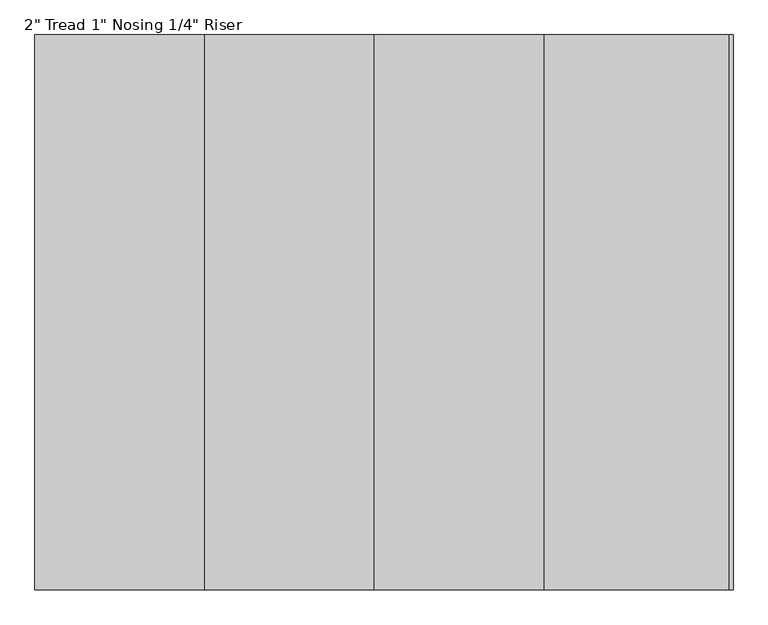
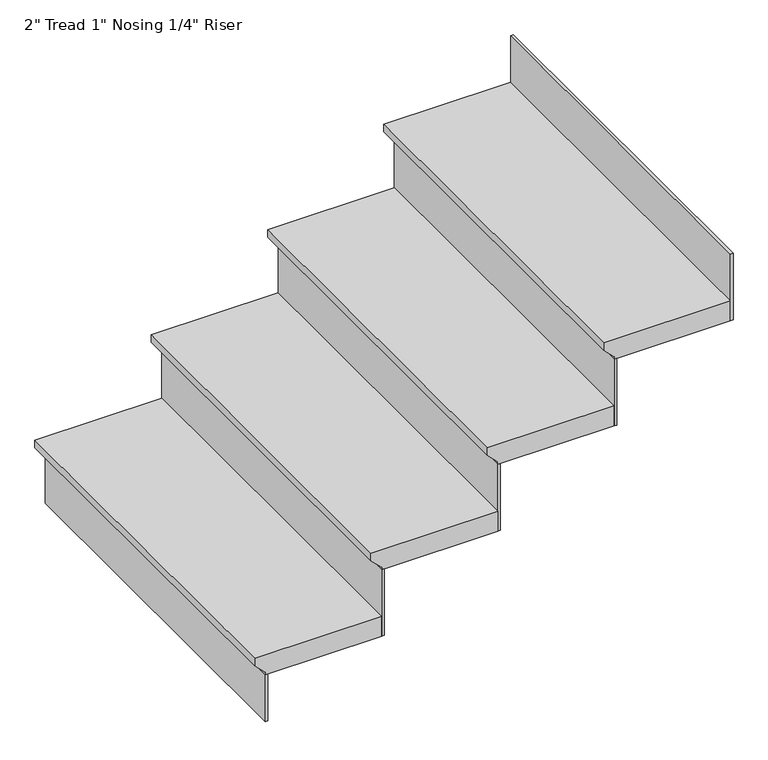
"""IFC4 building model written with IfcOpenShell, lengths in millimetres: stair flight geometry."""

from ifc_helpers import new_model, si_unit, origin, place, context, project, spatial, faceted_brep, source, transform, mapped, element, save


def stair_flight_1d7161dd(model_context):
    return source(origin(), model_context, "Body", "Brep", [
        faceted_brep([(-8719.8399968, 10473.3610583, 150.2833333), (-8719.8399968, 10473.3610583, 169.3333333), (-8719.8399968, 11387.7610583, 169.3333333), (-8719.8399968, 11387.7610583, 150.2833333), (-8694.4399968, 10473.3610583, 124.8833333), (-8694.4399968, 11387.7610583, 124.8833333), (-8415.0399968, 10473.3610583, 169.3333333), (-8415.0399968, 11387.7610583, 169.3333333), (-8694.4399968, 11387.7610583, 118.5333333), (-8415.0399968, 11387.7610583, 118.5333333), (-8415.0399968, 10473.3610583, 118.5333333), (-8694.4399968, 10473.3610583, 118.5333333)], [[[0, 1, 2, 3]], [[4, 0, 3, 5]], [[2, 1, 6, 7]], [[8, 9, 10, 11]], [[2, 7, 9, 8, 5, 3]], [[8, 11, 4, 5]], [[6, 1, 0, 4, 11, 10]], [[7, 6, 10, 9]]]),
        faceted_brep([(-8694.4399968, 10473.3610583, 118.5333333), (-8694.4399968, 10473.3610583, 0.0), (-8688.0899968, 10473.3610583, 0.0), (-8688.0899968, 10473.3610583, 118.5333333), (-8694.4399968, 11387.7610583, 118.5333333), (-8688.0899968, 11387.7610583, 118.5333333), (-8688.0899968, 11387.7610583, 0.0), (-8694.4399968, 11387.7610583, 0.0)], [[[0, 1, 2, 3]], [[4, 5, 6, 7]], [[1, 0, 4, 7]], [[2, 1, 7, 6]], [[3, 2, 6, 5]], [[0, 3, 5, 4]]]),
        faceted_brep([(-8415.0399968, 10473.3610583, 287.8666667), (-8415.0399968, 10473.3610583, 118.5333333), (-8408.6899968, 10473.3610583, 118.5333333), (-8408.6899968, 10473.3610583, 287.8666667), (-8415.0399968, 11387.7610583, 287.8666667), (-8408.6899968, 11387.7610583, 287.8666667), (-8408.6899968, 11387.7610583, 118.5333333), (-8415.0399968, 11387.7610583, 118.5333333)], [[[0, 1, 2, 3]], [[4, 5, 6, 7]], [[1, 0, 4, 7]], [[2, 1, 7, 6]], [[3, 2, 6, 5]], [[0, 3, 5, 4]]]),
        faceted_brep([(-8440.4399968, 11387.7610583, 338.6666667), (-8440.4399968, 10473.3610583, 338.6666667), (-8135.6399968, 10473.3610583, 338.6666667), (-8135.6399968, 11387.7610583, 338.6666667), (-8415.0399968, 11387.7610583, 287.8666667), (-8135.6399968, 11387.7610583, 287.8666667), (-8135.6399968, 10473.3610583, 287.8666667), (-8415.0399968, 10473.3610583, 287.8666667), (-8415.0399968, 11387.7610583, 294.2166667), (-8440.4399968, 11387.7610583, 319.6166667), (-8415.0399968, 10473.3610583, 294.2166667), (-8440.4399968, 10473.3610583, 319.6166667)], [[[0, 1, 2, 3]], [[4, 5, 6, 7]], [[0, 3, 5, 4, 8, 9]], [[4, 7, 10, 8]], [[2, 1, 11, 10, 7, 6]], [[3, 2, 6, 5]], [[11, 1, 0, 9]], [[10, 11, 9, 8]]]),
        faceted_brep([(-8135.6399968, 10473.3610583, 457.2), (-8135.6399968, 10473.3610583, 287.8666667), (-8129.2899968, 10473.3610583, 287.8666667), (-8129.2899968, 10473.3610583, 457.2), (-8135.6399968, 11387.7610583, 457.2), (-8129.2899968, 11387.7610583, 457.2), (-8129.2899968, 11387.7610583, 287.8666667), (-8135.6399968, 11387.7610583, 287.8666667)], [[[0, 1, 2, 3]], [[4, 5, 6, 7]], [[1, 0, 4, 7]], [[2, 1, 7, 6]], [[3, 2, 6, 5]], [[0, 3, 5, 4]]]),
        faceted_brep([(-8161.0399968, 11387.7610583, 508.0), (-8161.0399968, 10473.3610583, 508.0), (-7856.2399968, 10473.3610583, 508.0), (-7856.2399968, 11387.7610583, 508.0), (-8135.6399968, 11387.7610583, 457.2), (-7856.2399968, 11387.7610583, 457.2), (-7856.2399968, 10473.3610583, 457.2), (-8135.6399968, 10473.3610583, 457.2), (-8135.6399968, 11387.7610583, 463.55), (-8161.0399968, 11387.7610583, 488.95), (-8135.6399968, 10473.3610583, 463.55), (-8161.0399968, 10473.3610583, 488.95)], [[[0, 1, 2, 3]], [[4, 5, 6, 7]], [[0, 3, 5, 4, 8, 9]], [[4, 7, 10, 8]], [[2, 1, 11, 10, 7, 6]], [[3, 2, 6, 5]], [[11, 1, 0, 9]], [[10, 11, 9, 8]]]),
        faceted_brep([(-7576.8399968, 10473.3610583, 795.8666667), (-7576.8399968, 10473.3610583, 626.5333333), (-7570.4899968, 10473.3610583, 626.5333333), (-7570.4899968, 10473.3610583, 795.8666667), (-7576.8399968, 11387.7610583, 795.8666667), (-7570.4899968, 11387.7610583, 795.8666667), (-7570.4899968, 11387.7610583, 626.5333333), (-7576.8399968, 11387.7610583, 626.5333333)], [[[0, 1, 2, 3]], [[4, 5, 6, 7]], [[1, 0, 4, 7]], [[2, 1, 7, 6]], [[3, 2, 6, 5]], [[0, 3, 5, 4]]]),
        faceted_brep([(-7856.2399968, 10473.3610583, 626.5333333), (-7856.2399968, 10473.3610583, 457.2), (-7849.8899968, 10473.3610583, 457.2), (-7849.8899968, 10473.3610583, 626.5333333), (-7856.2399968, 11387.7610583, 626.5333333), (-7849.8899968, 11387.7610583, 626.5333333), (-7849.8899968, 11387.7610583, 457.2), (-7856.2399968, 11387.7610583, 457.2)], [[[0, 1, 2, 3]], [[4, 5, 6, 7]], [[1, 0, 4, 7]], [[2, 1, 7, 6]], [[3, 2, 6, 5]], [[0, 3, 5, 4]]]),
        faceted_brep([(-7576.8399968, 11387.7610583, 677.3333333), (-7602.2399968, 11387.7610583, 677.3333333), (-7881.6399968, 11387.7610583, 677.3333333), (-7881.6399968, 10473.3610583, 677.3333333), (-7576.8399968, 10473.3610583, 677.3333333), (-7602.2399968, 11387.7610583, 626.5333333), (-7576.8399968, 11387.7610583, 626.5333333), (-7576.8399968, 10473.3610583, 626.5333333), (-7856.2399968, 10473.3610583, 626.5333333), (-7856.2399968, 11387.7610583, 626.5333333), (-7856.2399968, 11387.7610583, 632.8833333), (-7881.6399968, 11387.7610583, 658.2833333), (-7856.2399968, 10473.3610583, 632.8833333), (-7881.6399968, 10473.3610583, 658.2833333)], [[[0, 1, 2, 3, 4]], [[5, 6, 7, 8, 9]], [[1, 0, 6, 5]], [[2, 1, 5, 9, 10, 11]], [[9, 8, 12, 10]], [[4, 3, 13, 12, 8, 7]], [[0, 4, 7, 6]], [[13, 3, 2, 11]], [[12, 13, 11, 10]]]),
    ])


if __name__ == "__main__":
    model = new_model("IFC4")
    model_context = context("Model", 3, world=origin())
    ifc_project = project(units=[si_unit("LENGTHUNIT", "METRE", prefix="MILLI")], contexts=[model_context])
    site = spatial("IfcSite", under=ifc_project)
    building = spatial("IfcBuilding", under=site)
    placement = place(None, origin())
    stair_flight_shape = stair_flight_1d7161dd(model_context)
    element("IfcStairFlight", 1, ObjectType="2\" Tread 1\" Nosing 1/4\" Riser", at=placement, inside=building, context=model_context, shape_type="MappedRepresentation", body=[
        mapped(stair_flight_shape, transform((0.0, 0.0, 0.0), x_axis=(1.0, 0.0, 0.0), y_axis=(0.0, 1.0, 0.0), z_axis=(0.0, 0.0, 1.0))),
    ])
    save(model, "model.ifc")
